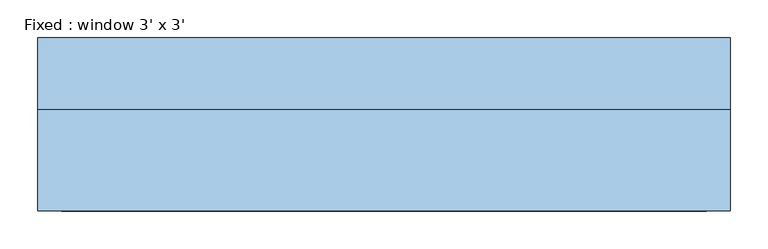
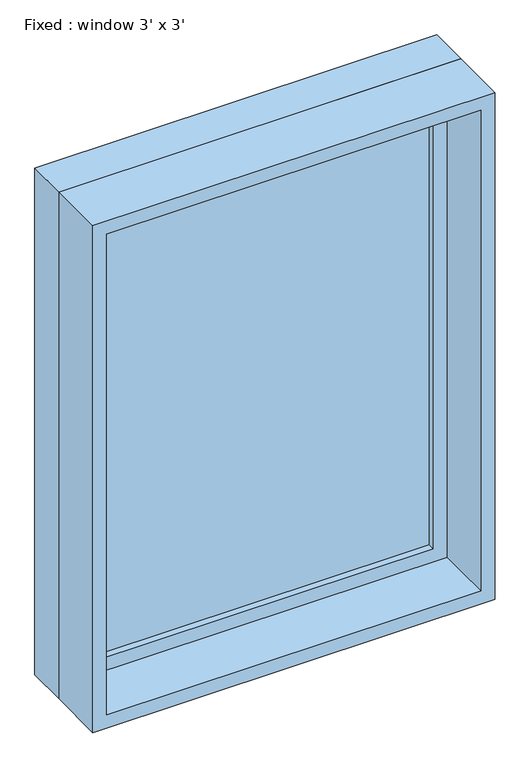
"""IFC4 building model written with IfcOpenShell, lengths in millimetres: window geometry, Fixed : window 3' x 3'."""

from ifc_helpers import new_model, si_unit, frame, origin, place, context, project, spatial, polyline, outline, extrude, source, transform, mapped, element, save


def fixed_window_3_x_3_dcb239d8(model_context):
    return source(origin(), model_context, "Body", "SweptSolid", [
        extrude(outline(polyline([(355.6, 34.925), (-431.8, 34.925), (-431.8, 47.625), (355.6, 47.625), (355.6, 34.925)])), frame((0.0, 0.0, 977.9), z_axis=(0.0, 0.0, 1.0), x_axis=(1.0, 0.0, 0.0)), (0.0, 0.0, 1.0), 1092.2),
        extrude(outline(polyline([(2114.55, -476.25), (933.45, -476.25), (933.45, 400.05), (2114.55, 400.05), (2114.55, -476.25)]), holes=[polyline([(2070.1, -431.8), (2070.1, 355.6), (977.9, 355.6), (977.9, -431.8), (2070.1, -431.8)])]), frame((0.0, 19.05, 0.0), z_axis=(0.0, 1.0, 0.0), x_axis=(0.0, 0.0, 1.0)), (0.0, 0.0, 1.0), 44.45),
        extrude(outline(polyline([(2133.6, -495.3), (914.4, -495.3), (914.4, 419.1), (2133.6, 419.1), (2133.6, -495.3)]), holes=[polyline([(2101.85, -463.55), (2101.85, 387.35), (946.15, 387.35), (946.15, -463.55), (2101.85, -463.55)])]), frame((0.0, -114.3, 0.0), z_axis=(0.0, 1.0, 0.0), x_axis=(0.0, 0.0, 1.0)), (0.0, 0.0, 1.0), 133.35),
        extrude(outline(polyline([(2133.6, 419.1), (2133.6, -495.3), (914.4, -495.3), (914.4, 419.1), (2133.6, 419.1)]), holes=[polyline([(2114.55, 400.05), (933.45, 400.05), (933.45, -476.25), (2114.55, -476.25), (2114.55, 400.05)])]), frame((0.0, 19.05, 0.0), z_axis=(0.0, 1.0, 0.0), x_axis=(0.0, 0.0, 1.0)), (0.0, 0.0, 1.0), 95.25),
    ])


if __name__ == "__main__":
    model = new_model("IFC4")
    model_context = context("Model", 3, world=origin())
    ifc_project = project(units=[si_unit("LENGTHUNIT", "METRE", prefix="MILLI")], contexts=[model_context])
    site = spatial("IfcSite", under=ifc_project)
    building = spatial("IfcBuilding", under=site)
    placement = place(None, origin())
    fixed_window_3_x_3_shape = fixed_window_3_x_3_dcb239d8(model_context)
    element("IfcWindow", 1, ObjectType="Fixed : window 3' x 3'", at=placement, inside=building, context=model_context, shape_type="MappedRepresentation", body=[
        mapped(fixed_window_3_x_3_shape, transform((0.0, 0.0, 0.0), x_axis=(1.0, 0.0, 0.0), y_axis=(0.0, 1.0, 0.0), z_axis=(0.0, 0.0, 1.0))),
    ])
    save(model, "model.ifc")

# Revit data of these elements
# Type "Fixed : window 3' x 3'"
#   Type Mark = "18"
#   Construction Type Id = "GSP4R"
#   Assembly Code = "B2020100"
#   Analytic Construction = "1/8 in Pilkington single glazing"
#   Visual Light Transmittance = 0.9
#   Solar Heat Gain Coefficient = 0.78
#   Heat Transfer Coefficient (U) = 0.6496 BTU/(h·ft²·°F)
#   Height = 4' - 0"
#   Default Sill Height = 3' - 0"
#   Width = 3' - 0"
#   Window Inset = 0' - 2"
#   Define Thermal Properties by = 1
#   Glass Pane Material = Glass
#   Sash Material = Sash
#   Wall Closure = (empty or 0)
# Element 1 (IfcWindow, "Fixed : window 3' x 3'")
#   Materials on its faces: "Sash", "Glass"
# Materials
#   "Glass": class "Glass", colour RGB 0 128 192, transparency 0.75, Description = "Soda Lime Glass", Cost = 0
#   "Sash": class "Wood", colour RGB 224 178 126, transparency 0, Cost = 0
